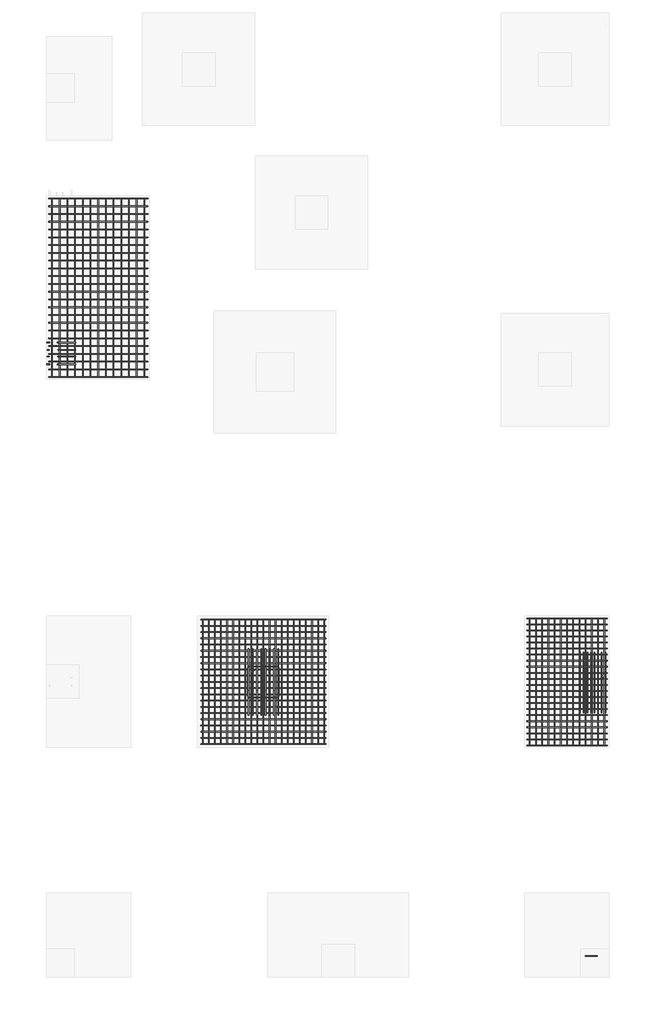
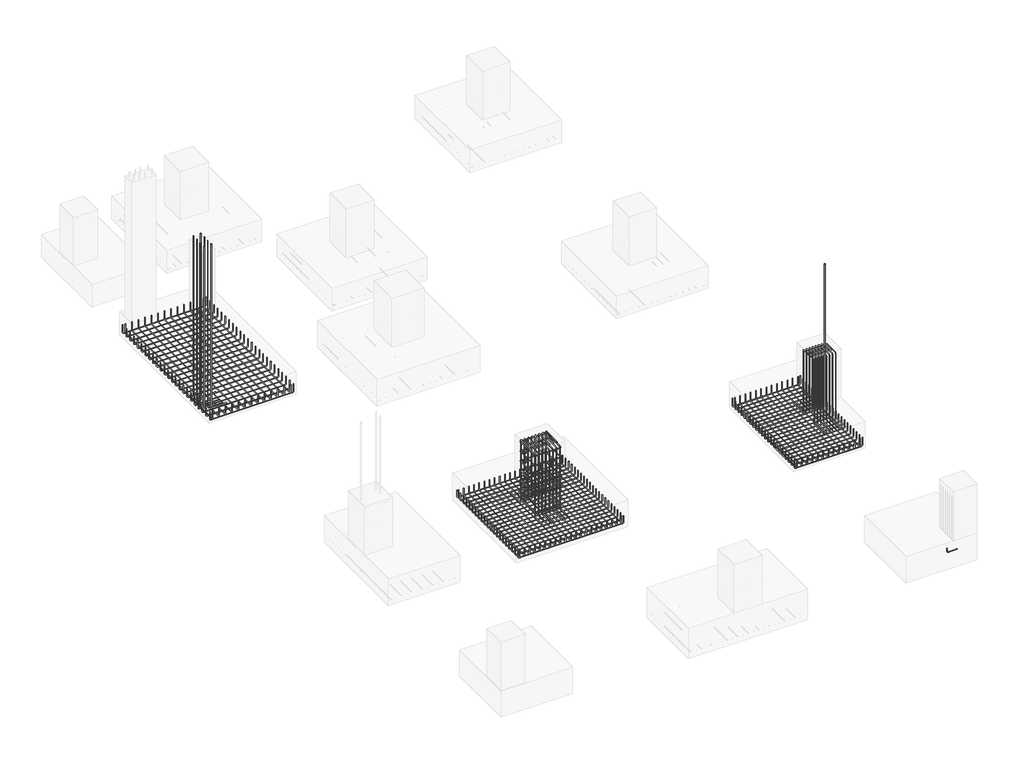
# One storey, part 3 of 6: 17 reinforcing bars.
"""IFC4 building model written with IfcOpenShell, lengths in millimetres."""

from ifc_helpers import new_model, si_unit, point, frame, origin, place, context, project, spatial, polyline, circle_curve, trimmed, segment, composite_curve, source, transform, mapped, element, save
from ifc_brep_helpers import swept_disk

model = new_model("IFC4")

# Units and contexts
model_context = context("Model", 3, world=origin())
ifc_project = project(units=[si_unit("LENGTHUNIT", "METRE", prefix="MILLI")], contexts=[model_context])

# Site, building, storey
site = spatial("IfcSite", under=ifc_project)
building = spatial("IfcBuilding", under=site)
storey = spatial("IfcBuildingStorey", under=building, Elevation=0.0)

# Reinforcing bars
placement = place(None, origin())
reinforcing_bar_shape = source(origin(), model_context, "Body", "SolidModel", [
    swept_disk(composite_curve([segment(polyline([(158081.8232069, -104044.3007776, -331.0), (158081.8232069, -104044.3007776, -473.4)]), True, "CONTINUOUS"), segment(trimmed(circle_curve(frame((158106.8232069, -104044.3007776, -473.4), z_axis=(0.0, -1.0, 0.0), x_axis=(-25.0, 0.0, 0.0)), 25.0), [point((158081.8232069, -104044.3007776, -473.4))], [point((158106.8232069, -104044.3007776, -498.4))], True, "CARTESIAN"), True, "CONTINUOUS"), segment(polyline([(158106.8232069, -104044.3007776, -498.4), (159358.4232069, -104044.3007776, -498.4)]), True, "CONTINUOUS"), segment(trimmed(circle_curve(frame((159358.4232069, -104044.3007776, -473.4), z_axis=(0.0, -1.0, 0.0), x_axis=(0.0, 0.0, -25.0)), 25.0), [point((159358.4232069, -104044.3007776, -498.4))], [point((159383.4232069, -104044.3007776, -473.4))], True, "CARTESIAN"), True, "CONTINUOUS"), segment(polyline([(159383.4232069, -104044.3007776, -473.4), (159383.4232069, -104044.3007776, -331.0)]), True, "CONTINUOUS")], self_intersect=False), 5.0),
])
element("IfcReinforcingBar", 1, at=placement, inside=storey, context=model_context, shape_type="MappedRepresentation", body=[
    mapped(reinforcing_bar_shape, transform((0.0, 0.0, 0.0), x_axis=(1.0, 0.0, 0.0), y_axis=(0.0, 1.0, 0.0), z_axis=(0.0, 0.0, 1.0))),
    mapped(reinforcing_bar_shape, transform((0.0, -98.2666667, 0.0), x_axis=(1.0, 0.0, 0.0), y_axis=(0.0, 1.0, 0.0), z_axis=(0.0, 0.0, 1.0))),
    mapped(reinforcing_bar_shape, transform((0.0, -196.5333333, 0.0), x_axis=(1.0, 0.0, 0.0), y_axis=(0.0, 1.0, 0.0), z_axis=(0.0, 0.0, 1.0))),
    mapped(reinforcing_bar_shape, transform((0.0, -294.8, 0.0), x_axis=(1.0, 0.0, 0.0), y_axis=(0.0, 1.0, 0.0), z_axis=(0.0, 0.0, 1.0))),
    mapped(reinforcing_bar_shape, transform((0.0, -393.0666667, 0.0), x_axis=(1.0, 0.0, 0.0), y_axis=(0.0, 1.0, 0.0), z_axis=(0.0, 0.0, 1.0))),
    mapped(reinforcing_bar_shape, transform((0.0, -491.3333333, 0.0), x_axis=(1.0, 0.0, 0.0), y_axis=(0.0, 1.0, 0.0), z_axis=(0.0, 0.0, 1.0))),
    mapped(reinforcing_bar_shape, transform((0.0, -589.6, 0.0), x_axis=(1.0, 0.0, 0.0), y_axis=(0.0, 1.0, 0.0), z_axis=(0.0, 0.0, 1.0))),
    mapped(reinforcing_bar_shape, transform((0.0, -687.8666667, 0.0), x_axis=(1.0, 0.0, 0.0), y_axis=(0.0, 1.0, 0.0), z_axis=(0.0, 0.0, 1.0))),
    mapped(reinforcing_bar_shape, transform((0.0, -786.1333333, 0.0), x_axis=(1.0, 0.0, 0.0), y_axis=(0.0, 1.0, 0.0), z_axis=(0.0, 0.0, 1.0))),
    mapped(reinforcing_bar_shape, transform((0.0, -884.4, 0.0), x_axis=(1.0, 0.0, 0.0), y_axis=(0.0, 1.0, 0.0), z_axis=(0.0, 0.0, 1.0))),
    mapped(reinforcing_bar_shape, transform((0.0, -982.6666667, 0.0), x_axis=(1.0, 0.0, 0.0), y_axis=(0.0, 1.0, 0.0), z_axis=(0.0, 0.0, 1.0))),
    mapped(reinforcing_bar_shape, transform((0.0, -1080.9333333, 0.0), x_axis=(1.0, 0.0, 0.0), y_axis=(0.0, 1.0, 0.0), z_axis=(0.0, 0.0, 1.0))),
    mapped(reinforcing_bar_shape, transform((0.0, -1179.2, 0.0), x_axis=(1.0, 0.0, 0.0), y_axis=(0.0, 1.0, 0.0), z_axis=(0.0, 0.0, 1.0))),
    mapped(reinforcing_bar_shape, transform((0.0, -1277.4666667, 0.0), x_axis=(1.0, 0.0, 0.0), y_axis=(0.0, 1.0, 0.0), z_axis=(0.0, 0.0, 1.0))),
    mapped(reinforcing_bar_shape, transform((0.0, -1375.7333333, 0.0), x_axis=(1.0, 0.0, 0.0), y_axis=(0.0, 1.0, 0.0), z_axis=(0.0, 0.0, 1.0))),
    mapped(reinforcing_bar_shape, transform((0.0, -1474.0, 0.0), x_axis=(1.0, 0.0, 0.0), y_axis=(0.0, 1.0, 0.0), z_axis=(0.0, 0.0, 1.0))),
    mapped(reinforcing_bar_shape, transform((0.0, -1572.2666667, 0.0), x_axis=(1.0, 0.0, 0.0), y_axis=(0.0, 1.0, 0.0), z_axis=(0.0, 0.0, 1.0))),
    mapped(reinforcing_bar_shape, transform((0.0, -1670.5333333, 0.0), x_axis=(1.0, 0.0, 0.0), y_axis=(0.0, 1.0, 0.0), z_axis=(0.0, 0.0, 1.0))),
    mapped(reinforcing_bar_shape, transform((0.0, -1768.8, 0.0), x_axis=(1.0, 0.0, 0.0), y_axis=(0.0, 1.0, 0.0), z_axis=(0.0, 0.0, 1.0))),
    mapped(reinforcing_bar_shape, transform((0.0, -1867.0666667, 0.0), x_axis=(1.0, 0.0, 0.0), y_axis=(0.0, 1.0, 0.0), z_axis=(0.0, 0.0, 1.0))),
    mapped(reinforcing_bar_shape, transform((0.0, -1965.3333333, 0.0), x_axis=(1.0, 0.0, 0.0), y_axis=(0.0, 1.0, 0.0), z_axis=(0.0, 0.0, 1.0))),
    mapped(reinforcing_bar_shape, transform((0.0, -2063.6, 0.0), x_axis=(1.0, 0.0, 0.0), y_axis=(0.0, 1.0, 0.0), z_axis=(0.0, 0.0, 1.0))),
])
reinforcing_bar_2_shape = source(origin(), model_context, "Body", "SolidModel", [
    swept_disk(composite_curve([segment(polyline([(158127.2678893, -106107.9007776, -331.0), (158127.2678893, -106107.9007776, -473.4)]), True, "CONTINUOUS"), segment(trimmed(circle_curve(frame((158127.2678893, -106082.9007776, -473.4), z_axis=(1.0, 0.0, 0.0), x_axis=(0.0, -25.0, 0.0)), 25.0), [point((158127.2678893, -106107.9007776, -473.4))], [point((158127.2678893, -106082.9007776, -498.4))], True, "CARTESIAN"), True, "CONTINUOUS"), segment(polyline([(158127.2678893, -106082.9007776, -498.4), (158127.2678893, -104069.3007776, -498.4)]), True, "CONTINUOUS"), segment(trimmed(circle_curve(frame((158127.2678893, -104069.3007776, -473.4), z_axis=(1.0, 0.0, 0.0), x_axis=(0.0, 0.0, -25.0)), 25.0), [point((158127.2678893, -104069.3007776, -498.4))], [point((158127.2678893, -104044.3007776, -473.4))], True, "CARTESIAN"), True, "CONTINUOUS"), segment(polyline([(158127.2678893, -104044.3007776, -473.4), (158127.2678893, -104044.3007776, -331.0)]), True, "CONTINUOUS")], self_intersect=False), 5.0),
])
element("IfcReinforcingBar", 2, at=placement, inside=storey, context=model_context, shape_type="MappedRepresentation", body=[
    mapped(reinforcing_bar_2_shape, transform((0.0, 0.0, 0.0), x_axis=(1.0, 0.0, 0.0), y_axis=(0.0, 1.0, 0.0), z_axis=(0.0, 0.0, 1.0))),
    mapped(reinforcing_bar_2_shape, transform((100.9434332, 0.0, 0.0), x_axis=(1.0, 0.0, 0.0), y_axis=(0.0, 1.0, 0.0), z_axis=(0.0, 0.0, 1.0))),
    mapped(reinforcing_bar_2_shape, transform((201.8868664, 0.0, 0.0), x_axis=(1.0, 0.0, 0.0), y_axis=(0.0, 1.0, 0.0), z_axis=(0.0, 0.0, 1.0))),
    mapped(reinforcing_bar_2_shape, transform((302.8302996, 0.0, 0.0), x_axis=(1.0, 0.0, 0.0), y_axis=(0.0, 1.0, 0.0), z_axis=(0.0, 0.0, 1.0))),
    mapped(reinforcing_bar_2_shape, transform((403.7737328, 0.0, 0.0), x_axis=(1.0, 0.0, 0.0), y_axis=(0.0, 1.0, 0.0), z_axis=(0.0, 0.0, 1.0))),
    mapped(reinforcing_bar_2_shape, transform((504.717166, 0.0, 0.0), x_axis=(1.0, 0.0, 0.0), y_axis=(0.0, 1.0, 0.0), z_axis=(0.0, 0.0, 1.0))),
    mapped(reinforcing_bar_2_shape, transform((605.6605992, 0.0, 0.0), x_axis=(1.0, 0.0, 0.0), y_axis=(0.0, 1.0, 0.0), z_axis=(0.0, 0.0, 1.0))),
    mapped(reinforcing_bar_2_shape, transform((706.6040324, 0.0, 0.0), x_axis=(1.0, 0.0, 0.0), y_axis=(0.0, 1.0, 0.0), z_axis=(0.0, 0.0, 1.0))),
    mapped(reinforcing_bar_2_shape, transform((807.5474656, 0.0, 0.0), x_axis=(1.0, 0.0, 0.0), y_axis=(0.0, 1.0, 0.0), z_axis=(0.0, 0.0, 1.0))),
    mapped(reinforcing_bar_2_shape, transform((908.4908989, 0.0, 0.0), x_axis=(1.0, 0.0, 0.0), y_axis=(0.0, 1.0, 0.0), z_axis=(0.0, 0.0, 1.0))),
    mapped(reinforcing_bar_2_shape, transform((1009.4343321, 0.0, 0.0), x_axis=(1.0, 0.0, 0.0), y_axis=(0.0, 1.0, 0.0), z_axis=(0.0, 0.0, 1.0))),
    mapped(reinforcing_bar_2_shape, transform((1110.3777653, 0.0, 0.0), x_axis=(1.0, 0.0, 0.0), y_axis=(0.0, 1.0, 0.0), z_axis=(0.0, 0.0, 1.0))),
    mapped(reinforcing_bar_2_shape, transform((1211.3211985, 0.0, 0.0), x_axis=(1.0, 0.0, 0.0), y_axis=(0.0, 1.0, 0.0), z_axis=(0.0, 0.0, 1.0))),
])
reinforcing_bar_3_shape = source(origin(), model_context, "Body", "SolidModel", [
    swept_disk(composite_curve([segment(polyline([(152786.2805846, -104064.3007776, -331.0), (152786.2805846, -104064.3007776, -453.4)]), True, "CONTINUOUS"), segment(trimmed(circle_curve(frame((152811.2805846, -104064.3007776, -453.4), z_axis=(0.0, -1.0, 0.0), x_axis=(-25.0, 0.0, 0.0)), 25.0), [point((152786.2805846, -104064.3007776, -453.4))], [point((152811.2805846, -104064.3007776, -478.4))], True, "CARTESIAN"), True, "CONTINUOUS"), segment(polyline([(152811.2805846, -104064.3007776, -478.4), (154784.8805846, -104064.3007776, -478.4)]), True, "CONTINUOUS"), segment(trimmed(circle_curve(frame((154784.8805846, -104064.3007776, -453.4), z_axis=(0.0, -1.0, 0.0), x_axis=(0.0, 0.0, -25.0)), 25.0), [point((154784.8805846, -104064.3007776, -478.4))], [point((154809.8805846, -104064.3007776, -453.4))], True, "CARTESIAN"), True, "CONTINUOUS"), segment(polyline([(154809.8805846, -104064.3007776, -453.4), (154809.8805846, -104064.3007776, -331.0)]), True, "CONTINUOUS")], self_intersect=False), 5.0),
])
element("IfcReinforcingBar", 3, at=placement, inside=storey, context=model_context, shape_type="MappedRepresentation", body=[
    mapped(reinforcing_bar_3_shape, transform((0.0, 0.0, 0.0), x_axis=(1.0, 0.0, 0.0), y_axis=(0.0, 1.0, 0.0), z_axis=(0.0, 0.0, 1.0))),
    mapped(reinforcing_bar_3_shape, transform((0.0, -101.18, 0.0), x_axis=(1.0, 0.0, 0.0), y_axis=(0.0, 1.0, 0.0), z_axis=(0.0, 0.0, 1.0))),
    mapped(reinforcing_bar_3_shape, transform((0.0, -202.36, 0.0), x_axis=(1.0, 0.0, 0.0), y_axis=(0.0, 1.0, 0.0), z_axis=(0.0, 0.0, 1.0))),
    mapped(reinforcing_bar_3_shape, transform((0.0, -303.54, 0.0), x_axis=(1.0, 0.0, 0.0), y_axis=(0.0, 1.0, 0.0), z_axis=(0.0, 0.0, 1.0))),
    mapped(reinforcing_bar_3_shape, transform((0.0, -404.72, 0.0), x_axis=(1.0, 0.0, 0.0), y_axis=(0.0, 1.0, 0.0), z_axis=(0.0, 0.0, 1.0))),
    mapped(reinforcing_bar_3_shape, transform((0.0, -505.9, 0.0), x_axis=(1.0, 0.0, 0.0), y_axis=(0.0, 1.0, 0.0), z_axis=(0.0, 0.0, 1.0))),
    mapped(reinforcing_bar_3_shape, transform((0.0, -607.08, 0.0), x_axis=(1.0, 0.0, 0.0), y_axis=(0.0, 1.0, 0.0), z_axis=(0.0, 0.0, 1.0))),
    mapped(reinforcing_bar_3_shape, transform((0.0, -708.26, 0.0), x_axis=(1.0, 0.0, 0.0), y_axis=(0.0, 1.0, 0.0), z_axis=(0.0, 0.0, 1.0))),
    mapped(reinforcing_bar_3_shape, transform((0.0, -809.44, 0.0), x_axis=(1.0, 0.0, 0.0), y_axis=(0.0, 1.0, 0.0), z_axis=(0.0, 0.0, 1.0))),
    mapped(reinforcing_bar_3_shape, transform((0.0, -910.62, 0.0), x_axis=(1.0, 0.0, 0.0), y_axis=(0.0, 1.0, 0.0), z_axis=(0.0, 0.0, 1.0))),
    mapped(reinforcing_bar_3_shape, transform((0.0, -1011.8, 0.0), x_axis=(1.0, 0.0, 0.0), y_axis=(0.0, 1.0, 0.0), z_axis=(0.0, 0.0, 1.0))),
    mapped(reinforcing_bar_3_shape, transform((0.0, -1112.98, 0.0), x_axis=(1.0, 0.0, 0.0), y_axis=(0.0, 1.0, 0.0), z_axis=(0.0, 0.0, 1.0))),
    mapped(reinforcing_bar_3_shape, transform((0.0, -1214.16, 0.0), x_axis=(1.0, 0.0, 0.0), y_axis=(0.0, 1.0, 0.0), z_axis=(0.0, 0.0, 1.0))),
    mapped(reinforcing_bar_3_shape, transform((0.0, -1315.34, 0.0), x_axis=(1.0, 0.0, 0.0), y_axis=(0.0, 1.0, 0.0), z_axis=(0.0, 0.0, 1.0))),
    mapped(reinforcing_bar_3_shape, transform((0.0, -1416.52, 0.0), x_axis=(1.0, 0.0, 0.0), y_axis=(0.0, 1.0, 0.0), z_axis=(0.0, 0.0, 1.0))),
    mapped(reinforcing_bar_3_shape, transform((0.0, -1517.7, 0.0), x_axis=(1.0, 0.0, 0.0), y_axis=(0.0, 1.0, 0.0), z_axis=(0.0, 0.0, 1.0))),
    mapped(reinforcing_bar_3_shape, transform((0.0, -1618.88, 0.0), x_axis=(1.0, 0.0, 0.0), y_axis=(0.0, 1.0, 0.0), z_axis=(0.0, 0.0, 1.0))),
    mapped(reinforcing_bar_3_shape, transform((0.0, -1720.06, 0.0), x_axis=(1.0, 0.0, 0.0), y_axis=(0.0, 1.0, 0.0), z_axis=(0.0, 0.0, 1.0))),
    mapped(reinforcing_bar_3_shape, transform((0.0, -1821.24, 0.0), x_axis=(1.0, 0.0, 0.0), y_axis=(0.0, 1.0, 0.0), z_axis=(0.0, 0.0, 1.0))),
    mapped(reinforcing_bar_3_shape, transform((0.0, -1922.42, 0.0), x_axis=(1.0, 0.0, 0.0), y_axis=(0.0, 1.0, 0.0), z_axis=(0.0, 0.0, 1.0))),
    mapped(reinforcing_bar_3_shape, transform((0.0, -2023.6, 0.0), x_axis=(1.0, 0.0, 0.0), y_axis=(0.0, 1.0, 0.0), z_axis=(0.0, 0.0, 1.0))),
])
reinforcing_bar_4_shape = source(origin(), model_context, "Body", "SolidModel", [
    swept_disk(composite_curve([segment(polyline([(152812.8758289, -106087.9007776, -331.0), (152812.8758289, -106087.9007776, -453.4)]), True, "CONTINUOUS"), segment(trimmed(circle_curve(frame((152812.8758289, -106062.9007776, -453.4), z_axis=(1.0, 0.0, 0.0), x_axis=(0.0, -25.0, 0.0)), 25.0), [point((152812.8758289, -106087.9007776, -453.4))], [point((152812.8758289, -106062.9007776, -478.4))], True, "CARTESIAN"), True, "CONTINUOUS"), segment(polyline([(152812.8758289, -106062.9007776, -478.4), (152812.8758289, -104089.3007776, -478.4)]), True, "CONTINUOUS"), segment(trimmed(circle_curve(frame((152812.8758289, -104089.3007776, -453.4), z_axis=(1.0, 0.0, 0.0), x_axis=(0.0, 0.0, -25.0)), 25.0), [point((152812.8758289, -104089.3007776, -478.4))], [point((152812.8758289, -104064.3007776, -453.4))], True, "CARTESIAN"), True, "CONTINUOUS"), segment(polyline([(152812.8758289, -104064.3007776, -453.4), (152812.8758289, -104064.3007776, -331.0)]), True, "CONTINUOUS")], self_intersect=False), 5.0),
])
element("IfcReinforcingBar", 4, at=placement, inside=storey, context=model_context, shape_type="MappedRepresentation", body=[
    mapped(reinforcing_bar_4_shape, transform((0.0, 0.0, 0.0), x_axis=(1.0, 0.0, 0.0), y_axis=(0.0, 1.0, 0.0), z_axis=(0.0, 0.0, 1.0))),
    mapped(reinforcing_bar_4_shape, transform((98.6274824, 0.0, 0.0), x_axis=(1.0, 0.0, 0.0), y_axis=(0.0, 1.0, 0.0), z_axis=(0.0, 0.0, 1.0))),
    mapped(reinforcing_bar_4_shape, transform((197.2549649, 0.0, 0.0), x_axis=(1.0, 0.0, 0.0), y_axis=(0.0, 1.0, 0.0), z_axis=(0.0, 0.0, 1.0))),
    mapped(reinforcing_bar_4_shape, transform((295.8824473, 0.0, 0.0), x_axis=(1.0, 0.0, 0.0), y_axis=(0.0, 1.0, 0.0), z_axis=(0.0, 0.0, 1.0))),
    mapped(reinforcing_bar_4_shape, transform((394.5099298, 0.0, 0.0), x_axis=(1.0, 0.0, 0.0), y_axis=(0.0, 1.0, 0.0), z_axis=(0.0, 0.0, 1.0))),
    mapped(reinforcing_bar_4_shape, transform((493.1374122, 0.0, 0.0), x_axis=(1.0, 0.0, 0.0), y_axis=(0.0, 1.0, 0.0), z_axis=(0.0, 0.0, 1.0))),
    mapped(reinforcing_bar_4_shape, transform((591.7648947, 0.0, 0.0), x_axis=(1.0, 0.0, 0.0), y_axis=(0.0, 1.0, 0.0), z_axis=(0.0, 0.0, 1.0))),
    mapped(reinforcing_bar_4_shape, transform((690.3923771, 0.0, 0.0), x_axis=(1.0, 0.0, 0.0), y_axis=(0.0, 1.0, 0.0), z_axis=(0.0, 0.0, 1.0))),
    mapped(reinforcing_bar_4_shape, transform((789.0198596, 0.0, 0.0), x_axis=(1.0, 0.0, 0.0), y_axis=(0.0, 1.0, 0.0), z_axis=(0.0, 0.0, 1.0))),
    mapped(reinforcing_bar_4_shape, transform((887.647342, 0.0, 0.0), x_axis=(1.0, 0.0, 0.0), y_axis=(0.0, 1.0, 0.0), z_axis=(0.0, 0.0, 1.0))),
    mapped(reinforcing_bar_4_shape, transform((986.2748245, 0.0, 0.0), x_axis=(1.0, 0.0, 0.0), y_axis=(0.0, 1.0, 0.0), z_axis=(0.0, 0.0, 1.0))),
    mapped(reinforcing_bar_4_shape, transform((1084.9023069, 0.0, 0.0), x_axis=(1.0, 0.0, 0.0), y_axis=(0.0, 1.0, 0.0), z_axis=(0.0, 0.0, 1.0))),
    mapped(reinforcing_bar_4_shape, transform((1183.5297894, 0.0, 0.0), x_axis=(1.0, 0.0, 0.0), y_axis=(0.0, 1.0, 0.0), z_axis=(0.0, 0.0, 1.0))),
    mapped(reinforcing_bar_4_shape, transform((1282.1572718, 0.0, 0.0), x_axis=(1.0, 0.0, 0.0), y_axis=(0.0, 1.0, 0.0), z_axis=(0.0, 0.0, 1.0))),
    mapped(reinforcing_bar_4_shape, transform((1380.7847543, 0.0, 0.0), x_axis=(1.0, 0.0, 0.0), y_axis=(0.0, 1.0, 0.0), z_axis=(0.0, 0.0, 1.0))),
    mapped(reinforcing_bar_4_shape, transform((1479.4122367, 0.0, 0.0), x_axis=(1.0, 0.0, 0.0), y_axis=(0.0, 1.0, 0.0), z_axis=(0.0, 0.0, 1.0))),
    mapped(reinforcing_bar_4_shape, transform((1578.0397191, 0.0, 0.0), x_axis=(1.0, 0.0, 0.0), y_axis=(0.0, 1.0, 0.0), z_axis=(0.0, 0.0, 1.0))),
    mapped(reinforcing_bar_4_shape, transform((1676.6672016, 0.0, 0.0), x_axis=(1.0, 0.0, 0.0), y_axis=(0.0, 1.0, 0.0), z_axis=(0.0, 0.0, 1.0))),
    mapped(reinforcing_bar_4_shape, transform((1775.294684, 0.0, 0.0), x_axis=(1.0, 0.0, 0.0), y_axis=(0.0, 1.0, 0.0), z_axis=(0.0, 0.0, 1.0))),
    mapped(reinforcing_bar_4_shape, transform((1873.9221665, 0.0, 0.0), x_axis=(1.0, 0.0, 0.0), y_axis=(0.0, 1.0, 0.0), z_axis=(0.0, 0.0, 1.0))),
    mapped(reinforcing_bar_4_shape, transform((1972.5496489, 0.0, 0.0), x_axis=(1.0, 0.0, 0.0), y_axis=(0.0, 1.0, 0.0), z_axis=(0.0, 0.0, 1.0))),
])
reinforcing_bar_5_shape = source(origin(), model_context, "Body", "SolidModel", [
    swept_disk(composite_curve([segment(polyline([(150309.4232069, -97224.4007776, -254.8), (150309.4232069, -97224.4007776, -397.2)]), True, "CONTINUOUS"), segment(trimmed(circle_curve(frame((150334.4232069, -97224.4007776, -397.2), z_axis=(0.0, -1.0, 0.0), x_axis=(-25.0, 0.0, 0.0)), 25.0), [point((150309.4232069, -97224.4007776, -397.2))], [point((150334.4232069, -97224.4007776, -422.2))], True, "CARTESIAN"), True, "CONTINUOUS"), segment(polyline([(150334.4232069, -97224.4007776, -422.2), (151890.8232069, -97224.4007776, -422.2)]), True, "CONTINUOUS"), segment(trimmed(circle_curve(frame((151890.8232069, -97224.4007776, -397.2), z_axis=(0.0, -1.0, 0.0), x_axis=(0.0, 0.0, -25.0)), 25.0), [point((151890.8232069, -97224.4007776, -422.2))], [point((151915.8232069, -97224.4007776, -397.2))], True, "CARTESIAN"), True, "CONTINUOUS"), segment(polyline([(151915.8232069, -97224.4007776, -397.2), (151915.8232069, -97224.4007776, -254.8)]), True, "CONTINUOUS")], self_intersect=False), 5.0),
])
element("IfcReinforcingBar", 5, at=placement, inside=storey, context=model_context, shape_type="MappedRepresentation", body=[
    mapped(reinforcing_bar_5_shape, transform((0.0, 0.0, 0.0), x_axis=(1.0, 0.0, 0.0), y_axis=(0.0, 1.0, 0.0), z_axis=(0.0, 0.0, 1.0))),
    mapped(reinforcing_bar_5_shape, transform((0.0, -126.1652174, 0.0), x_axis=(1.0, 0.0, 0.0), y_axis=(0.0, 1.0, 0.0), z_axis=(0.0, 0.0, 1.0))),
    mapped(reinforcing_bar_5_shape, transform((0.0, -252.3304348, 0.0), x_axis=(1.0, 0.0, 0.0), y_axis=(0.0, 1.0, 0.0), z_axis=(0.0, 0.0, 1.0))),
    mapped(reinforcing_bar_5_shape, transform((0.0, -378.4956522, 0.0), x_axis=(1.0, 0.0, 0.0), y_axis=(0.0, 1.0, 0.0), z_axis=(0.0, 0.0, 1.0))),
    mapped(reinforcing_bar_5_shape, transform((0.0, -504.6608696, 0.0), x_axis=(1.0, 0.0, 0.0), y_axis=(0.0, 1.0, 0.0), z_axis=(0.0, 0.0, 1.0))),
    mapped(reinforcing_bar_5_shape, transform((0.0, -630.826087, 0.0), x_axis=(1.0, 0.0, 0.0), y_axis=(0.0, 1.0, 0.0), z_axis=(0.0, 0.0, 1.0))),
    mapped(reinforcing_bar_5_shape, transform((0.0, -756.9913043, 0.0), x_axis=(1.0, 0.0, 0.0), y_axis=(0.0, 1.0, 0.0), z_axis=(0.0, 0.0, 1.0))),
    mapped(reinforcing_bar_5_shape, transform((0.0, -883.1565217, 0.0), x_axis=(1.0, 0.0, 0.0), y_axis=(0.0, 1.0, 0.0), z_axis=(0.0, 0.0, 1.0))),
    mapped(reinforcing_bar_5_shape, transform((0.0, -1009.3217391, 0.0), x_axis=(1.0, 0.0, 0.0), y_axis=(0.0, 1.0, 0.0), z_axis=(0.0, 0.0, 1.0))),
    mapped(reinforcing_bar_5_shape, transform((0.0, -1135.4869565, 0.0), x_axis=(1.0, 0.0, 0.0), y_axis=(0.0, 1.0, 0.0), z_axis=(0.0, 0.0, 1.0))),
    mapped(reinforcing_bar_5_shape, transform((0.0, -1261.6521739, 0.0), x_axis=(1.0, 0.0, 0.0), y_axis=(0.0, 1.0, 0.0), z_axis=(0.0, 0.0, 1.0))),
    mapped(reinforcing_bar_5_shape, transform((0.0, -1387.8173913, 0.0), x_axis=(1.0, 0.0, 0.0), y_axis=(0.0, 1.0, 0.0), z_axis=(0.0, 0.0, 1.0))),
    mapped(reinforcing_bar_5_shape, transform((0.0, -1513.9826087, 0.0), x_axis=(1.0, 0.0, 0.0), y_axis=(0.0, 1.0, 0.0), z_axis=(0.0, 0.0, 1.0))),
    mapped(reinforcing_bar_5_shape, transform((0.0, -1640.1478261, 0.0), x_axis=(1.0, 0.0, 0.0), y_axis=(0.0, 1.0, 0.0), z_axis=(0.0, 0.0, 1.0))),
    mapped(reinforcing_bar_5_shape, transform((0.0, -1766.3130435, 0.0), x_axis=(1.0, 0.0, 0.0), y_axis=(0.0, 1.0, 0.0), z_axis=(0.0, 0.0, 1.0))),
    mapped(reinforcing_bar_5_shape, transform((0.0, -1892.4782609, 0.0), x_axis=(1.0, 0.0, 0.0), y_axis=(0.0, 1.0, 0.0), z_axis=(0.0, 0.0, 1.0))),
    mapped(reinforcing_bar_5_shape, transform((0.0, -2018.6434783, 0.0), x_axis=(1.0, 0.0, 0.0), y_axis=(0.0, 1.0, 0.0), z_axis=(0.0, 0.0, 1.0))),
    mapped(reinforcing_bar_5_shape, transform((0.0, -2144.8086957, 0.0), x_axis=(1.0, 0.0, 0.0), y_axis=(0.0, 1.0, 0.0), z_axis=(0.0, 0.0, 1.0))),
    mapped(reinforcing_bar_5_shape, transform((0.0, -2270.973913, 0.0), x_axis=(1.0, 0.0, 0.0), y_axis=(0.0, 1.0, 0.0), z_axis=(0.0, 0.0, 1.0))),
    mapped(reinforcing_bar_5_shape, transform((0.0, -2397.1391304, 0.0), x_axis=(1.0, 0.0, 0.0), y_axis=(0.0, 1.0, 0.0), z_axis=(0.0, 0.0, 1.0))),
    mapped(reinforcing_bar_5_shape, transform((0.0, -2523.3043478, 0.0), x_axis=(1.0, 0.0, 0.0), y_axis=(0.0, 1.0, 0.0), z_axis=(0.0, 0.0, 1.0))),
    mapped(reinforcing_bar_5_shape, transform((0.0, -2649.4695652, 0.0), x_axis=(1.0, 0.0, 0.0), y_axis=(0.0, 1.0, 0.0), z_axis=(0.0, 0.0, 1.0))),
    mapped(reinforcing_bar_5_shape, transform((0.0, -2775.6347826, 0.0), x_axis=(1.0, 0.0, 0.0), y_axis=(0.0, 1.0, 0.0), z_axis=(0.0, 0.0, 1.0))),
    mapped(reinforcing_bar_5_shape, transform((0.0, -2901.8, 0.0), x_axis=(1.0, 0.0, 0.0), y_axis=(0.0, 1.0, 0.0), z_axis=(0.0, 0.0, 1.0))),
])
reinforcing_bar_6_shape = source(origin(), model_context, "Body", "SolidModel", [
    swept_disk(composite_curve([segment(polyline([(150361.4391163, -100126.2007776, -254.8), (150361.4391163, -100126.2007776, -397.2)]), True, "CONTINUOUS"), segment(trimmed(circle_curve(frame((150361.4391163, -100101.2007776, -397.2), z_axis=(1.0, 0.0, 0.0), x_axis=(0.0, -25.0, 0.0)), 25.0), [point((150361.4391163, -100126.2007776, -397.2))], [point((150361.4391163, -100101.2007776, -422.2))], True, "CARTESIAN"), True, "CONTINUOUS"), segment(polyline([(150361.4391163, -100101.2007776, -422.2), (150361.4391163, -97249.4007776, -422.2)]), True, "CONTINUOUS"), segment(trimmed(circle_curve(frame((150361.4391163, -97249.4007776, -397.2), z_axis=(1.0, 0.0, 0.0), x_axis=(0.0, 0.0, -25.0)), 25.0), [point((150361.4391163, -97249.4007776, -422.2))], [point((150361.4391163, -97224.4007776, -397.2))], True, "CARTESIAN"), True, "CONTINUOUS"), segment(polyline([(150361.4391163, -97224.4007776, -397.2), (150361.4391163, -97224.4007776, -254.8)]), True, "CONTINUOUS")], self_intersect=False), 5.0),
])
element("IfcReinforcingBar", 6, at=placement, inside=storey, context=model_context, shape_type="MappedRepresentation", body=[
    mapped(reinforcing_bar_6_shape, transform((0.0, 0.0, 0.0), x_axis=(1.0, 0.0, 0.0), y_axis=(0.0, 1.0, 0.0), z_axis=(0.0, 0.0, 1.0))),
    mapped(reinforcing_bar_6_shape, transform((125.1036153, 0.0, 0.0), x_axis=(1.0, 0.0, 0.0), y_axis=(0.0, 1.0, 0.0), z_axis=(0.0, 0.0, 1.0))),
    mapped(reinforcing_bar_6_shape, transform((250.2072306, 0.0, 0.0), x_axis=(1.0, 0.0, 0.0), y_axis=(0.0, 1.0, 0.0), z_axis=(0.0, 0.0, 1.0))),
    mapped(reinforcing_bar_6_shape, transform((375.3108459, 0.0, 0.0), x_axis=(1.0, 0.0, 0.0), y_axis=(0.0, 1.0, 0.0), z_axis=(0.0, 0.0, 1.0))),
    mapped(reinforcing_bar_6_shape, transform((500.4144612, 0.0, 0.0), x_axis=(1.0, 0.0, 0.0), y_axis=(0.0, 1.0, 0.0), z_axis=(0.0, 0.0, 1.0))),
    mapped(reinforcing_bar_6_shape, transform((625.5180764, 0.0, 0.0), x_axis=(1.0, 0.0, 0.0), y_axis=(0.0, 1.0, 0.0), z_axis=(0.0, 0.0, 1.0))),
    mapped(reinforcing_bar_6_shape, transform((750.6216917, 0.0, 0.0), x_axis=(1.0, 0.0, 0.0), y_axis=(0.0, 1.0, 0.0), z_axis=(0.0, 0.0, 1.0))),
    mapped(reinforcing_bar_6_shape, transform((875.725307, 0.0, 0.0), x_axis=(1.0, 0.0, 0.0), y_axis=(0.0, 1.0, 0.0), z_axis=(0.0, 0.0, 1.0))),
    mapped(reinforcing_bar_6_shape, transform((1000.8289223, 0.0, 0.0), x_axis=(1.0, 0.0, 0.0), y_axis=(0.0, 1.0, 0.0), z_axis=(0.0, 0.0, 1.0))),
    mapped(reinforcing_bar_6_shape, transform((1125.9325376, 0.0, 0.0), x_axis=(1.0, 0.0, 0.0), y_axis=(0.0, 1.0, 0.0), z_axis=(0.0, 0.0, 1.0))),
    mapped(reinforcing_bar_6_shape, transform((1251.0361529, 0.0, 0.0), x_axis=(1.0, 0.0, 0.0), y_axis=(0.0, 1.0, 0.0), z_axis=(0.0, 0.0, 1.0))),
    mapped(reinforcing_bar_6_shape, transform((1376.1397682, 0.0, 0.0), x_axis=(1.0, 0.0, 0.0), y_axis=(0.0, 1.0, 0.0), z_axis=(0.0, 0.0, 1.0))),
    mapped(reinforcing_bar_6_shape, transform((1501.2433835, 0.0, 0.0), x_axis=(1.0, 0.0, 0.0), y_axis=(0.0, 1.0, 0.0), z_axis=(0.0, 0.0, 1.0))),
])
reinforcing_bar_7_shape = source(origin(), model_context, "Body", "SolidModel", [
    swept_disk(composite_curve([segment(polyline([(154039.8805846, -105213.6465608, 908.7608209), (154039.8805846, -104870.3465608, 908.7608209)]), True, "CONTINUOUS"), segment(trimmed(circle_curve(frame((154039.8805846, -104870.3465608, 883.7608209), z_axis=(-1.0, 0.0, 0.0), x_axis=(0.0, 0.0, 25.0)), 25.0), [point((154039.8805846, -104870.3465608, 908.7608209))], [point((154039.8805846, -104845.3465608, 883.7608209))], True, "CARTESIAN"), True, "CONTINUOUS"), segment(polyline([(154039.8805846, -104845.3465608, 883.7608209), (154039.8805846, -104845.3465608, -355.2891791)]), True, "CONTINUOUS"), segment(trimmed(circle_curve(frame((154039.8805846, -104820.3465608, -355.2891791), z_axis=(1.0, 0.0, 0.0), x_axis=(0.0, -25.0, 0.0)), 25.0), [point((154039.8805846, -104845.3465608, -355.2891791))], [point((154039.8805846, -104820.3465608, -380.2891791))], True, "CARTESIAN"), True, "CONTINUOUS"), segment(polyline([(154039.8805846, -104820.3465608, -380.2891791), (154039.8805846, -104540.5465608, -380.2891791)]), True, "CONTINUOUS")], self_intersect=False), 5.0),
])
element("IfcReinforcingBar", 7, at=placement, inside=storey, context=model_context, shape_type="MappedRepresentation", body=[
    mapped(reinforcing_bar_7_shape, transform((0.0, 0.0, 0.0), x_axis=(1.0, 0.0, 0.0), y_axis=(0.0, 1.0, 0.0), z_axis=(0.0, 0.0, 1.0))),
    mapped(reinforcing_bar_7_shape, transform((-69.0857143, 0.0, 0.0), x_axis=(1.0, 0.0, 0.0), y_axis=(0.0, 1.0, 0.0), z_axis=(0.0, 0.0, 1.0))),
    mapped(reinforcing_bar_7_shape, transform((-138.1714286, 0.0, 0.0), x_axis=(1.0, 0.0, 0.0), y_axis=(0.0, 1.0, 0.0), z_axis=(0.0, 0.0, 1.0))),
    mapped(reinforcing_bar_7_shape, transform((-207.2571429, 0.0, 0.0), x_axis=(1.0, 0.0, 0.0), y_axis=(0.0, 1.0, 0.0), z_axis=(0.0, 0.0, 1.0))),
    mapped(reinforcing_bar_7_shape, transform((-276.3428571, 0.0, 0.0), x_axis=(1.0, 0.0, 0.0), y_axis=(0.0, 1.0, 0.0), z_axis=(0.0, 0.0, 1.0))),
    mapped(reinforcing_bar_7_shape, transform((-345.4285714, 0.0, 0.0), x_axis=(1.0, 0.0, 0.0), y_axis=(0.0, 1.0, 0.0), z_axis=(0.0, 0.0, 1.0))),
    mapped(reinforcing_bar_7_shape, transform((-414.5142857, 0.0, 0.0), x_axis=(1.0, 0.0, 0.0), y_axis=(0.0, 1.0, 0.0), z_axis=(0.0, 0.0, 1.0))),
    mapped(reinforcing_bar_7_shape, transform((-483.6, 0.0, 0.0), x_axis=(1.0, 0.0, 0.0), y_axis=(0.0, 1.0, 0.0), z_axis=(0.0, 0.0, 1.0))),
])
reinforcing_bar_8_shape = source(origin(), model_context, "Body", "SolidModel", [
    swept_disk(composite_curve([segment(polyline([(154039.8805846, -104944.9049943, 882.2485592), (154039.8805846, -105288.2049943, 882.2485592)]), True, "CONTINUOUS"), segment(trimmed(circle_curve(frame((154039.8805846, -105288.2049943, 857.2485592), z_axis=(1.0, 0.0, 0.0), x_axis=(0.0, 0.0, 25.0)), 25.0), [point((154039.8805846, -105288.2049943, 882.2485592))], [point((154039.8805846, -105313.2049943, 857.2485592))], True, "CARTESIAN"), True, "CONTINUOUS"), segment(polyline([(154039.8805846, -105313.2049943, 857.2485592), (154039.8805846, -105313.2049943, -355.2891791)]), True, "CONTINUOUS"), segment(trimmed(circle_curve(frame((154039.8805846, -105338.2049943, -355.2891791), z_axis=(-1.0, 0.0, 0.0), x_axis=(0.0, 25.0, 0.0)), 25.0), [point((154039.8805846, -105313.2049943, -355.2891791))], [point((154039.8805846, -105338.2049943, -380.2891791))], True, "CARTESIAN"), True, "CONTINUOUS"), segment(polyline([(154039.8805846, -105338.2049943, -380.2891791), (154039.8805846, -105618.0049943, -380.2891791)]), True, "CONTINUOUS")], self_intersect=False), 5.0),
])
element("IfcReinforcingBar", 8, at=placement, inside=storey, context=model_context, shape_type="MappedRepresentation", body=[
    mapped(reinforcing_bar_8_shape, transform((0.0, 0.0, 0.0), x_axis=(1.0, 0.0, 0.0), y_axis=(0.0, 1.0, 0.0), z_axis=(0.0, 0.0, 1.0))),
    mapped(reinforcing_bar_8_shape, transform((-69.0857143, 0.0, 0.0), x_axis=(1.0, 0.0, 0.0), y_axis=(0.0, 1.0, 0.0), z_axis=(0.0, 0.0, 1.0))),
    mapped(reinforcing_bar_8_shape, transform((-138.1714286, 0.0, 0.0), x_axis=(1.0, 0.0, 0.0), y_axis=(0.0, 1.0, 0.0), z_axis=(0.0, 0.0, 1.0))),
    mapped(reinforcing_bar_8_shape, transform((-207.2571429, 0.0, 0.0), x_axis=(1.0, 0.0, 0.0), y_axis=(0.0, 1.0, 0.0), z_axis=(0.0, 0.0, 1.0))),
    mapped(reinforcing_bar_8_shape, transform((-276.3428571, 0.0, 0.0), x_axis=(1.0, 0.0, 0.0), y_axis=(0.0, 1.0, 0.0), z_axis=(0.0, 0.0, 1.0))),
    mapped(reinforcing_bar_8_shape, transform((-345.4285714, 0.0, 0.0), x_axis=(1.0, 0.0, 0.0), y_axis=(0.0, 1.0, 0.0), z_axis=(0.0, 0.0, 1.0))),
    mapped(reinforcing_bar_8_shape, transform((-414.5142857, 0.0, 0.0), x_axis=(1.0, 0.0, 0.0), y_axis=(0.0, 1.0, 0.0), z_axis=(0.0, 0.0, 1.0))),
    mapped(reinforcing_bar_8_shape, transform((-483.6, 0.0, 0.0), x_axis=(1.0, 0.0, 0.0), y_axis=(0.0, 1.0, 0.0), z_axis=(0.0, 0.0, 1.0))),
])
reinforcing_bar_9_shape = source(origin(), model_context, "Body", "SolidModel", [
    swept_disk(composite_curve([segment(polyline([(153617.485166, -104923.7896303, 857.221406), (153553.138449, -104859.4429132, 857.221406)]), True, "CONTINUOUS"), segment(trimmed(circle_curve(frame((153567.2805846, -104845.3007776, 857.221406), z_axis=(0.0, 0.0, -1.0), x_axis=(-14.14213560000644, -14.142135599991889, 0.0)), 20.0), [point((153553.138449, -104859.4429132, 857.221406))], [point((153567.2805846, -104825.3007776, 857.221406))], True, "CARTESIAN"), True, "CONTINUOUS"), segment(polyline([(153567.2805846, -104825.3007776, 857.221406), (154028.8805846, -104825.3007776, 857.221406)]), True, "CONTINUOUS"), segment(trimmed(circle_curve(frame((154028.8805846, -104845.3007776, 857.221406), z_axis=(0.0, 0.0, -1.0), x_axis=(0.0, 20.0, 0.0)), 20.0), [point((154028.8805846, -104825.3007776, 857.221406))], [point((154048.8805846, -104845.3007776, 857.221406))], True, "CARTESIAN"), True, "CONTINUOUS"), segment(polyline([(154048.8805846, -104845.3007776, 857.221406), (154048.8805846, -105306.9007776, 857.221406)]), True, "CONTINUOUS"), segment(trimmed(circle_curve(frame((154028.8831278, -105306.9007776, 857.5403447), z_axis=(-0.015946935239925984, 0.0, -0.999872839543336), x_axis=(19.997456799988868, 0.0, -0.3189386999999897)), 20.0), [point((154048.8805846, -105306.9007776, 857.221406))], [point((154028.8831278, -105326.9007776, 857.5403447))], True, "CARTESIAN"), True, "CONTINUOUS"), segment(polyline([(154028.8831278, -105326.9007776, 857.5403447), (153567.2780414, -105326.9007776, 864.9024673)]), True, "CONTINUOUS"), segment(trimmed(circle_curve(frame((153567.2780414, -105306.9007776, 864.9024673), z_axis=(-0.015946935239925984, 0.0, -0.999872839543336), x_axis=(0.0, -20.0, 0.0)), 20.0), [point((153567.2780414, -105326.9007776, 864.9024673))], [point((153547.2805846, -105306.9007776, 865.221406))], True, "CARTESIAN"), True, "CONTINUOUS"), segment(polyline([(153547.2805846, -105306.9007776, 865.221406), (153547.2805846, -104845.3007776, 865.221406)]), True, "CONTINUOUS"), segment(trimmed(circle_curve(frame((153567.2805846, -104845.3007776, 865.221406), z_axis=(0.0, 0.0, -1.0), x_axis=(-20.0, 0.0, 0.0)), 20.0), [point((153547.2805846, -104845.3007776, 865.221406))], [point((153581.4227202, -104831.158642, 865.221406))], True, "CARTESIAN"), True, "CONTINUOUS"), segment(polyline([(153581.4227202, -104831.158642, 865.221406), (153645.7694373, -104895.505359, 865.221406)]), True, "CONTINUOUS")], self_intersect=False), 4.0),
])
element("IfcReinforcingBar", 9, at=placement, inside=storey, context=model_context, shape_type="MappedRepresentation", body=[
    mapped(reinforcing_bar_9_shape, transform((0.0, 0.0, 0.0), x_axis=(1.0, 0.0, 0.0), y_axis=(0.0, 1.0, 0.0), z_axis=(0.0, 0.0, 1.0))),
    mapped(reinforcing_bar_9_shape, transform((0.0, 0.0, -195.2892017), x_axis=(1.0, 0.0, 0.0), y_axis=(0.0, 1.0, 0.0), z_axis=(0.0, 0.0, 1.0))),
    mapped(reinforcing_bar_9_shape, transform((0.0, 0.0, -390.5784033), x_axis=(1.0, 0.0, 0.0), y_axis=(0.0, 1.0, 0.0), z_axis=(0.0, 0.0, 1.0))),
    mapped(reinforcing_bar_9_shape, transform((0.0, 0.0, -585.867605), x_axis=(1.0, 0.0, 0.0), y_axis=(0.0, 1.0, 0.0), z_axis=(0.0, 0.0, 1.0))),
    mapped(reinforcing_bar_9_shape, transform((0.0, 0.0, -781.1568067), x_axis=(1.0, 0.0, 0.0), y_axis=(0.0, 1.0, 0.0), z_axis=(0.0, 0.0, 1.0))),
    mapped(reinforcing_bar_9_shape, transform((0.0, 0.0, -976.4460083), x_axis=(1.0, 0.0, 0.0), y_axis=(0.0, 1.0, 0.0), z_axis=(0.0, 0.0, 1.0))),
    mapped(reinforcing_bar_9_shape, transform((0.0, 0.0, -1171.73521), x_axis=(1.0, 0.0, 0.0), y_axis=(0.0, 1.0, 0.0), z_axis=(0.0, 0.0, 1.0))),
])
reinforcing_bar_10_shape = source(origin(), model_context, "Body", "SolidModel", [
    swept_disk(composite_curve([segment(polyline([(150320.4232069, -99919.80313, 2970.0), (150320.4232069, -99919.80313, -279.5075398)]), True, "CONTINUOUS"), segment(trimmed(circle_curve(frame((150280.4232069, -99919.80313, -279.5075398), z_axis=(0.0, 1.0, 0.0), x_axis=(40.0, 0.0, 0.0)), 40.0), [point((150320.4232069, -99919.80313, -279.5075398))], [point((150280.4232069, -99919.80313, -319.5075398))], True, "CARTESIAN"), True, "CONTINUOUS"), segment(polyline([(150280.4232069, -99919.80313, -319.5075398), (150272.6509962, -99919.80313, -319.5075398)]), True, "CONTINUOUS")], self_intersect=False), 8.0),
])
element("IfcReinforcingBar", 10, at=placement, inside=storey, context=model_context, shape_type="MappedRepresentation", body=[
    mapped(reinforcing_bar_10_shape, transform((0.0, 0.0, 0.0), x_axis=(1.0, 0.0, 0.0), y_axis=(0.0, 1.0, 0.0), z_axis=(0.0, 0.0, 1.0))),
    mapped(reinforcing_bar_10_shape, transform((0.0, 356.2103887, 0.0), x_axis=(1.0, 0.0, 0.0), y_axis=(0.0, 1.0, 0.0), z_axis=(0.0, 0.0, 1.0))),
])
reinforcing_bar_11_shape = source(origin(), model_context, "Body", "SolidModel", [
    swept_disk(composite_curve([segment(polyline([(150457.0232069, -99919.80313, 2970.0), (150457.0232069, -99919.80313, -313.3122672)]), True, "CONTINUOUS"), segment(trimmed(circle_curve(frame((150497.0232069, -99919.80313, -313.3122672), z_axis=(0.0, -1.0, 0.0), x_axis=(-40.0, 0.0, 0.0)), 40.0), [point((150457.0232069, -99919.80313, -313.3122672))], [point((150497.0232069, -99919.80313, -353.3122672))], True, "CARTESIAN"), True, "CONTINUOUS"), segment(polyline([(150497.0232069, -99919.80313, -353.3122672), (150746.1407417, -99919.80313, -353.3122672)]), True, "CONTINUOUS")], self_intersect=False), 8.0),
])
element("IfcReinforcingBar", 11, at=placement, inside=storey, context=model_context, shape_type="MappedRepresentation", body=[
    mapped(reinforcing_bar_11_shape, transform((0.0, 0.0, 0.0), x_axis=(1.0, 0.0, 0.0), y_axis=(0.0, 1.0, 0.0), z_axis=(0.0, 0.0, 1.0))),
    mapped(reinforcing_bar_11_shape, transform((0.0, 356.2103887, 0.0), x_axis=(1.0, 0.0, 0.0), y_axis=(0.0, 1.0, 0.0), z_axis=(0.0, 0.0, 1.0))),
])
reinforcing_bar_12_shape = source(origin(), model_context, "Body", "SolidModel", [
    swept_disk(composite_curve([segment(polyline([(150316.4232069, -99794.1439514, 2970.0), (150316.4232069, -99794.1439514, -367.5403473)]), True, "CONTINUOUS"), segment(trimmed(circle_curve(frame((150296.4232069, -99794.1439514, -367.5403473), z_axis=(0.0, 1.0, 0.0), x_axis=(20.0, 0.0, 0.0)), 20.0), [point((150316.4232069, -99794.1439514, -367.5403473))], [point((150296.4232069, -99794.1439514, -387.5403473))], True, "CARTESIAN"), True, "CONTINUOUS"), segment(polyline([(150296.4232069, -99794.1439514, -387.5403473), (150284.34294, -99794.1439514, -387.5403473)]), True, "CONTINUOUS")], self_intersect=False), 4.0),
])
element("IfcReinforcingBar", 12, at=placement, inside=storey, context=model_context, shape_type="MappedRepresentation", body=[
    mapped(reinforcing_bar_12_shape, transform((0.0, 0.0, 0.0), x_axis=(1.0, 0.0, 0.0), y_axis=(0.0, 1.0, 0.0), z_axis=(0.0, 0.0, 1.0))),
    mapped(reinforcing_bar_12_shape, transform((0.0, 112.6188396, 0.0), x_axis=(1.0, 0.0, 0.0), y_axis=(0.0, 1.0, 0.0), z_axis=(0.0, 0.0, 1.0))),
])
reinforcing_bar_13_shape = source(origin(), model_context, "Body", "SolidModel", [
    swept_disk(composite_curve([segment(polyline([(150461.0232069, -99794.1439514, 2970.0), (150461.0232069, -99794.1439514, -407.761022)]), True, "CONTINUOUS"), segment(trimmed(circle_curve(frame((150481.0232069, -99794.1439514, -407.761022), z_axis=(0.0, -1.0, 0.0), x_axis=(-20.0, 0.0, 0.0)), 20.0), [point((150461.0232069, -99794.1439514, -407.761022))], [point((150481.0232069, -99794.1439514, -427.761022))], True, "CARTESIAN"), True, "CONTINUOUS"), segment(polyline([(150481.0232069, -99794.1439514, -427.761022), (150750.5716096, -99794.1439514, -427.761022)]), True, "CONTINUOUS")], self_intersect=False), 4.0),
])
element("IfcReinforcingBar", 13, at=placement, inside=storey, context=model_context, shape_type="MappedRepresentation", body=[
    mapped(reinforcing_bar_13_shape, transform((0.0, 0.0, 0.0), x_axis=(1.0, 0.0, 0.0), y_axis=(0.0, 1.0, 0.0), z_axis=(0.0, 0.0, 1.0))),
    mapped(reinforcing_bar_13_shape, transform((0.0, 112.6188396, 0.0), x_axis=(1.0, 0.0, 0.0), y_axis=(0.0, 1.0, 0.0), z_axis=(0.0, 0.0, 1.0))),
])
element("IfcReinforcingBar", 14, at=placement, inside=storey, context=model_context, shape_type="SolidModel", body=[
    swept_disk(composite_curve([segment(polyline([(159227.9232069, -109530.0339158, -462.4652155), (159056.4846071, -109530.0339158, -462.4652155)]), True, "CONTINUOUS"), segment(trimmed(circle_curve(frame((159056.4846071, -109530.0339158, -442.4652155), z_axis=(0.0, 1.0, 0.0), x_axis=(0.0, 0.0, -20.0)), 20.0), [point((159056.4846071, -109530.0339158, -462.4652155))], [point((159036.4846071, -109530.0339158, -442.4652155))], True, "CARTESIAN"), True, "CONTINUOUS"), segment(polyline([(159036.4846071, -109530.0339158, -442.4652155), (159036.4846071, -109530.0339158, -382.8549127)]), True, "CONTINUOUS")], self_intersect=False), 4.0),
])
reinforcing_bar_14_shape = source(origin(), model_context, "Body", "SolidModel", [
    swept_disk(composite_curve([segment(polyline([(158947.0232069, -104983.5351466, 899.6018913), (158947.0232069, -105252.1507776, 899.6018913)]), True, "CONTINUOUS"), segment(trimmed(circle_curve(frame((158947.0232069, -105252.1507776, 879.6018913), z_axis=(1.0, 0.0, 0.0), x_axis=(0.0, 0.0, 20.0)), 20.0), [point((158947.0232069, -105252.1507776, 899.6018913))], [point((158947.0232069, -105272.1507776, 879.6018913))], True, "CARTESIAN"), True, "CONTINUOUS"), segment(polyline([(158947.0232069, -105272.1507776, 879.6018913), (158947.0232069, -105272.1507776, -399.7898753)]), True, "CONTINUOUS"), segment(trimmed(circle_curve(frame((158947.0232069, -105292.1507776, -399.7898753), z_axis=(-1.0, 0.0, 0.0), x_axis=(0.0, 20.0, 0.0)), 20.0), [point((158947.0232069, -105272.1507776, -399.7898753))], [point((158947.0232069, -105292.1507776, -419.7898753))], True, "CARTESIAN"), True, "CONTINUOUS"), segment(polyline([(158947.0232069, -105292.1507776, -419.7898753), (158947.0232069, -105576.9507776, -419.7898753)]), True, "CONTINUOUS")], self_intersect=False), 4.0),
])
element("IfcReinforcingBar", 15, at=placement, inside=storey, context=model_context, shape_type="MappedRepresentation", body=[
    mapped(reinforcing_bar_14_shape, transform((0.0, 0.0, 0.0), x_axis=(1.0, 0.0, 0.0), y_axis=(0.0, 1.0, 0.0), z_axis=(0.0, 0.0, 1.0))),
    mapped(reinforcing_bar_14_shape, transform((58.4857143, 0.0, 0.0), x_axis=(1.0, 0.0, 0.0), y_axis=(0.0, 1.0, 0.0), z_axis=(0.0, 0.0, 1.0))),
    mapped(reinforcing_bar_14_shape, transform((116.9714286, 0.0, 0.0), x_axis=(1.0, 0.0, 0.0), y_axis=(0.0, 1.0, 0.0), z_axis=(0.0, 0.0, 1.0))),
    mapped(reinforcing_bar_14_shape, transform((175.4571429, 0.0, 0.0), x_axis=(1.0, 0.0, 0.0), y_axis=(0.0, 1.0, 0.0), z_axis=(0.0, 0.0, 1.0))),
    mapped(reinforcing_bar_14_shape, transform((233.9428571, 0.0, 0.0), x_axis=(1.0, 0.0, 0.0), y_axis=(0.0, 1.0, 0.0), z_axis=(0.0, 0.0, 1.0))),
    mapped(reinforcing_bar_14_shape, transform((292.4285714, 0.0, 0.0), x_axis=(1.0, 0.0, 0.0), y_axis=(0.0, 1.0, 0.0), z_axis=(0.0, 0.0, 1.0))),
    mapped(reinforcing_bar_14_shape, transform((350.9142857, 0.0, 0.0), x_axis=(1.0, 0.0, 0.0), y_axis=(0.0, 1.0, 0.0), z_axis=(0.0, 0.0, 1.0))),
    mapped(reinforcing_bar_14_shape, transform((409.4, 0.0, 0.0), x_axis=(1.0, 0.0, 0.0), y_axis=(0.0, 1.0, 0.0), z_axis=(0.0, 0.0, 1.0))),
])
reinforcing_bar_15_shape = source(origin(), model_context, "Body", "SolidModel", [
    swept_disk(composite_curve([segment(polyline([(159356.4232069, -105135.8908057, 877.0190747), (159356.4232069, -104920.9408057, 877.0190747)]), True, "CONTINUOUS"), segment(trimmed(circle_curve(frame((159356.4232069, -104920.9408057, 857.0190747), z_axis=(-1.0, 0.0, 0.0), x_axis=(0.0, 0.0, 20.0)), 20.0), [point((159356.4232069, -104920.9408057, 877.0190747))], [point((159356.4232069, -104900.9408057, 857.0190747))], True, "CARTESIAN"), True, "CONTINUOUS"), segment(polyline([(159356.4232069, -104900.9408057, 857.0190747), (159356.4232069, -104900.9408057, -392.0309253)]), True, "CONTINUOUS"), segment(trimmed(circle_curve(frame((159356.4232069, -104880.9408057, -392.0309253), z_axis=(1.0, 0.0, 0.0), x_axis=(0.0, -20.0, 0.0)), 20.0), [point((159356.4232069, -104900.9408057, -392.0309253))], [point((159356.4232069, -104880.9408057, -412.0309253))], True, "CARTESIAN"), True, "CONTINUOUS"), segment(polyline([(159356.4232069, -104880.9408057, -412.0309253), (159356.4232069, -104596.1408057, -412.0309253)]), True, "CONTINUOUS")], self_intersect=False), 4.0),
])
element("IfcReinforcingBar", 16, at=placement, inside=storey, context=model_context, shape_type="MappedRepresentation", body=[
    mapped(reinforcing_bar_15_shape, transform((0.0, 0.0, 0.0), x_axis=(1.0, 0.0, 0.0), y_axis=(0.0, 1.0, 0.0), z_axis=(0.0, 0.0, 1.0))),
    mapped(reinforcing_bar_15_shape, transform((-58.4857143, 0.0, 0.0), x_axis=(1.0, 0.0, 0.0), y_axis=(0.0, 1.0, 0.0), z_axis=(0.0, 0.0, 1.0))),
    mapped(reinforcing_bar_15_shape, transform((-116.9714286, 0.0, 0.0), x_axis=(1.0, 0.0, 0.0), y_axis=(0.0, 1.0, 0.0), z_axis=(0.0, 0.0, 1.0))),
    mapped(reinforcing_bar_15_shape, transform((-175.4571429, 0.0, 0.0), x_axis=(1.0, 0.0, 0.0), y_axis=(0.0, 1.0, 0.0), z_axis=(0.0, 0.0, 1.0))),
    mapped(reinforcing_bar_15_shape, transform((-233.9428571, 0.0, 0.0), x_axis=(1.0, 0.0, 0.0), y_axis=(0.0, 1.0, 0.0), z_axis=(0.0, 0.0, 1.0))),
    mapped(reinforcing_bar_15_shape, transform((-292.4285714, 0.0, 0.0), x_axis=(1.0, 0.0, 0.0), y_axis=(0.0, 1.0, 0.0), z_axis=(0.0, 0.0, 1.0))),
    mapped(reinforcing_bar_15_shape, transform((-350.9142857, 0.0, 0.0), x_axis=(1.0, 0.0, 0.0), y_axis=(0.0, 1.0, 0.0), z_axis=(0.0, 0.0, 1.0))),
    mapped(reinforcing_bar_15_shape, transform((-409.4, 0.0, 0.0), x_axis=(1.0, 0.0, 0.0), y_axis=(0.0, 1.0, 0.0), z_axis=(0.0, 0.0, 1.0))),
])
element("IfcReinforcingBar", 17, at=placement, inside=storey, context=model_context, shape_type="SolidModel", body=[
    swept_disk(composite_curve([segment(polyline([(159293.8800612, -105010.1439233, 2557.2891341), (159293.8800612, -105010.1439233, -382.0926147)]), True, "CONTINUOUS"), segment(trimmed(circle_curve(frame((159322.1643324, -104981.8596521, -382.0926147), z_axis=(0.70710678118641, -0.707106781186685, 0.0), x_axis=(-28.284271199983777, -28.28427119999833, 0.0)), 40.0), [point((159293.8800612, -105010.1439233, -382.0926147))], [point((159322.1643324, -104981.8596521, -422.0926147))], True, "CARTESIAN"), True, "CONTINUOUS"), segment(polyline([(159322.1643324, -104981.8596521, -422.0926147), (159365.2425559, -104938.7814286, -422.0926147)]), True, "CONTINUOUS")], self_intersect=False), 8.0),
])

save(model, "model.ifc")

# Revit data of these elements
# Elements 1, 2, 3, 4, 5, 6, 7, 8, 9, 10, 11, 12, 13, 14, 15, 16, 17 (IfcReinforcingBar)
#   Phase Created = New Construction
